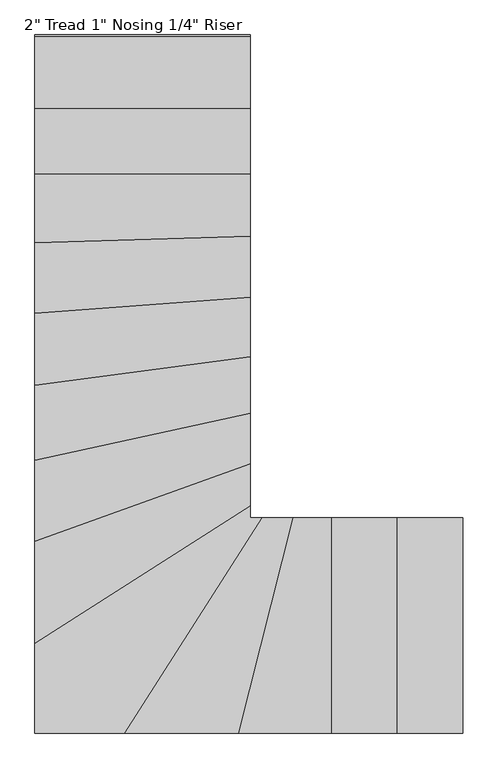
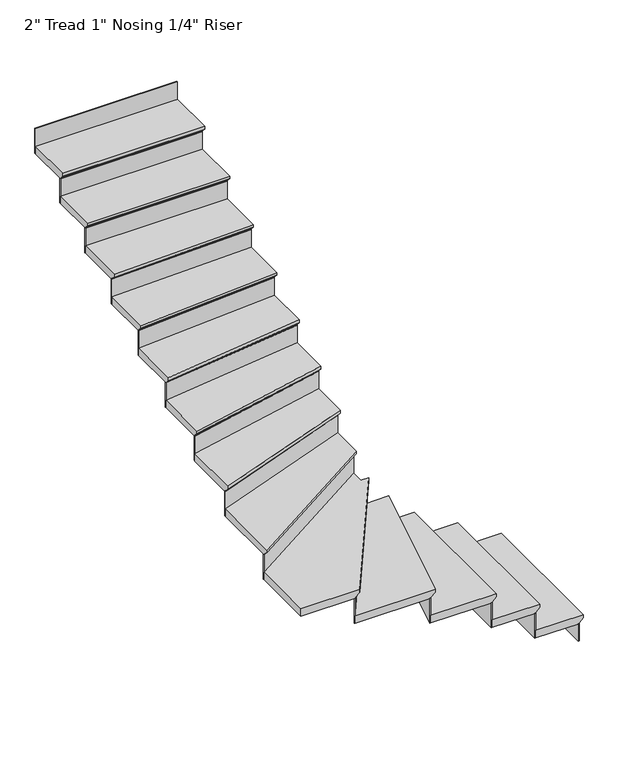
"""IFC4 building model written with IfcOpenShell, lengths in millimetres: stair flight geometry."""

from ifc_helpers import new_model, si_unit, origin, place, context, project, spatial, faceted_brep, source, transform, mapped, element, save


def stair_flight_28aaa101(model_context):
    return source(origin(), model_context, "Body", "Brep", [
        faceted_brep([(-12359.4290643, 4794.153629, 827.6166667), (-12359.4290643, 4794.153629, 846.6666667), (-12359.4290643, 3879.753629, 846.6666667), (-12359.4290643, 3879.753629, 827.6166667), (-12384.8290643, 4794.153629, 802.2166667), (-12384.8290643, 3879.753629, 802.2166667), (-12664.2290643, 4794.153629, 846.6666667), (-12664.2290643, 3879.753629, 846.6666667), (-12384.8290643, 3879.753629, 795.8666667), (-12664.2290643, 3879.753629, 795.8666667), (-12664.2290643, 4794.153629, 795.8666667), (-12384.8290643, 4794.153629, 795.8666667)], [[[0, 1, 2, 3]], [[4, 0, 3, 5]], [[2, 1, 6, 7]], [[8, 9, 10, 11]], [[2, 7, 9, 8, 5, 3]], [[8, 11, 4, 5]], [[6, 1, 0, 4, 11, 10]], [[7, 6, 10, 9]]]),
        faceted_brep([(-12384.8290643, 4794.153629, 795.8666667), (-12384.8290643, 4794.153629, 677.3333333), (-12391.1790643, 4794.153629, 677.3333333), (-12391.1790643, 4794.153629, 795.8666667), (-12384.8290643, 3879.753629, 795.8666667), (-12391.1790643, 3879.753629, 795.8666667), (-12391.1790643, 3879.753629, 677.3333333), (-12384.8290643, 3879.753629, 677.3333333)], [[[0, 1, 2, 3]], [[4, 5, 6, 7]], [[1, 0, 4, 7]], [[2, 1, 7, 6]], [[3, 2, 6, 5]], [[0, 3, 5, 4]]]),
        faceted_brep([(-12664.2290643, 4794.153629, 965.2), (-12664.2290643, 4794.153629, 795.8666667), (-12670.5790643, 4794.153629, 795.8666667), (-12670.5790643, 4794.153629, 965.2), (-12664.2290643, 3879.753629, 965.2), (-12670.5790643, 3879.753629, 965.2), (-12670.5790643, 3879.753629, 795.8666667), (-12664.2290643, 3879.753629, 795.8666667)], [[[0, 1, 2, 3]], [[4, 5, 6, 7]], [[1, 0, 4, 7]], [[2, 1, 7, 6]], [[3, 2, 6, 5]], [[0, 3, 5, 4]]]),
        faceted_brep([(-12638.8290643, 3879.753629, 1016.0), (-12638.8290643, 4794.153629, 1016.0), (-12943.6290643, 4794.153629, 1016.0), (-12943.6290643, 3879.753629, 1016.0), (-12664.2290643, 3879.753629, 965.2), (-12943.6290643, 3879.753629, 965.2), (-12943.6290643, 4794.153629, 965.2), (-12664.2290643, 4794.153629, 965.2), (-12664.2290643, 3879.753629, 971.55), (-12638.8290643, 3879.753629, 996.95), (-12664.2290643, 4794.153629, 971.55), (-12638.8290643, 4794.153629, 996.95)], [[[0, 1, 2, 3]], [[4, 5, 6, 7]], [[0, 3, 5, 4, 8, 9]], [[4, 7, 10, 8]], [[2, 1, 11, 10, 7, 6]], [[3, 2, 6, 5]], [[11, 1, 0, 9]], [[10, 11, 9, 8]]]),
        faceted_brep([(-12943.6290643, 4794.153629, 1134.5333333), (-12943.6290643, 4794.153629, 965.2), (-12949.9790643, 4794.153629, 965.2), (-12949.9790643, 4794.153629, 1134.5333333), (-12943.6290643, 3879.753629, 1134.5333333), (-12949.9790643, 3879.753629, 1134.5333333), (-12949.9790643, 3879.753629, 965.2), (-12943.6290643, 3879.753629, 965.2)], [[[0, 1, 2, 3]], [[4, 5, 6, 7]], [[1, 0, 4, 7]], [[2, 1, 7, 6]], [[3, 2, 6, 5]], [[0, 3, 5, 4]]]),
        faceted_brep([(-12918.2290643, 3879.753629, 1185.3333333), (-12918.2290643, 4794.153629, 1185.3333333), (-13108.3340982, 4794.153629, 1185.3333333), (-13339.3197748, 3879.753629, 1185.3333333), (-12943.6290643, 3879.753629, 1134.5333333), (-13339.3197748, 3879.753629, 1134.5333333), (-13108.3340982, 4794.153629, 1134.5333333), (-12943.6290643, 4794.153629, 1134.5333333), (-12943.6290643, 3879.753629, 1140.8833333), (-12918.2290643, 3879.753629, 1166.2833333), (-12943.6290643, 4794.153629, 1140.8833333), (-12918.2290643, 4794.153629, 1166.2833333)], [[[0, 1, 2, 3]], [[4, 5, 6, 7]], [[0, 3, 5, 4, 8, 9]], [[4, 7, 10, 8]], [[2, 1, 11, 10, 7, 6]], [[3, 2, 6, 5]], [[11, 1, 0, 9]], [[10, 11, 9, 8]]]),
        faceted_brep([(-13108.3340982, 4794.153629, 1303.8666667), (-13108.3340982, 4794.153629, 1134.5333333), (-13114.8835662, 4794.153629, 1134.5333333), (-13114.8835662, 4794.153629, 1303.8666667), (-13339.3197748, 3879.753629, 1303.8666667), (-13345.8692428, 3879.753629, 1303.8666667), (-13345.8692428, 3879.753629, 1134.5333333), (-13339.3197748, 3879.753629, 1134.5333333)], [[[0, 1, 2, 3]], [[4, 5, 6, 7]], [[1, 0, 4, 7]], [[2, 1, 7, 6]], [[3, 2, 6, 5]], [[0, 3, 5, 4]]]),
        faceted_brep([(-13313.1219026, 3879.753629, 1354.6666667), (-13082.136226, 4794.153629, 1354.6666667), (-13242.6016872, 4794.153629, 1354.6666667), (-13827.2011226, 3879.753629, 1354.6666667), (-13339.3197748, 3879.753629, 1303.8666667), (-13827.2011226, 3879.753629, 1303.8666667), (-13242.6016872, 4794.153629, 1303.8666667), (-13108.3340982, 4794.153629, 1303.8666667), (-13339.3197748, 3879.753629, 1310.2166667), (-13313.1219026, 3879.753629, 1335.6166667), (-13108.3340982, 4794.153629, 1310.2166667), (-13082.136226, 4794.153629, 1335.6166667)], [[[0, 1, 2, 3]], [[4, 5, 6, 7]], [[0, 3, 5, 4, 8, 9]], [[4, 7, 10, 8]], [[2, 1, 11, 10, 7, 6]], [[3, 2, 6, 5]], [[11, 1, 0, 9]], [[10, 11, 9, 8]]]),
        faceted_brep([(-13242.6016872, 4794.153629, 1473.2), (-13242.6016872, 4794.153629, 1303.8666667), (-13250.1385176, 4794.153629, 1303.8666667), (-13250.1385176, 4794.153629, 1473.2), (-13827.2011226, 3879.753629, 1473.2), (-13834.737953, 3879.753629, 1473.2), (-13834.737953, 3879.753629, 1303.8666667), (-13827.2011226, 3879.753629, 1303.8666667)], [[[0, 1, 2, 3]], [[4, 5, 6, 7]], [[1, 0, 4, 7]], [[2, 1, 7, 6]], [[3, 2, 6, 5]], [[0, 3, 5, 4]]]),
        faceted_brep([(-14177.7660538, 4290.6132035, 1524.0), (-14177.7660538, 3879.753629, 1524.0), (-13797.053801, 3879.753629, 1524.0), (-13212.4543656, 4794.153629, 1524.0), (-13263.3660538, 4794.153629, 1524.0), (-13263.3660538, 4875.2126389, 1524.0), (-14177.7660538, 3879.753629, 1473.2), (-14177.7660538, 4290.6132035, 1473.2), (-13263.3660538, 4875.2126389, 1473.2), (-13263.3660538, 4794.153629, 1473.2), (-13242.6016872, 4794.153629, 1473.2), (-13827.2011226, 3879.753629, 1473.2), (-13242.6016872, 4794.153629, 1479.55), (-13827.2011226, 3879.753629, 1479.55), (-13212.4543656, 4794.153629, 1504.95), (-13797.053801, 3879.753629, 1504.95)], [[[0, 1, 2, 3, 4, 5]], [[6, 7, 8, 9, 10, 11]], [[1, 0, 7, 6]], [[11, 10, 12, 13]], [[4, 3, 14, 12, 10, 9]], [[0, 5, 8, 7]], [[14, 3, 2, 15]], [[12, 14, 15, 13]], [[2, 1, 6, 11, 13, 15]], [[5, 4, 9, 8]]]),
        faceted_brep([(-13263.3660538, 4875.2126389, 1642.5333333), (-13263.3660538, 4875.2126389, 1473.2), (-13263.3660538, 4882.7494693, 1473.2), (-13263.3660538, 4882.7494693, 1642.5333333), (-14177.7660538, 4290.6132035, 1642.5333333), (-14177.7660538, 4298.1500339, 1642.5333333), (-14177.7660538, 4298.1500339, 1473.2), (-14177.7660538, 4290.6132035, 1473.2)], [[[0, 1, 2, 3]], [[4, 5, 6, 7]], [[1, 0, 4, 7]], [[2, 1, 7, 6]], [[3, 2, 6, 5]], [[0, 3, 5, 4]]]),
        faceted_brep([(-14177.7660538, 4260.4658819, 1693.3333333), (-13263.3660538, 4845.0653173, 1693.3333333), (-13263.3660538, 5051.1689508, 1693.3333333), (-14177.7660538, 4722.592446, 1693.3333333), (-14177.7660538, 4290.6132035, 1642.5333333), (-14177.7660538, 4722.592446, 1642.5333333), (-13263.3660538, 5051.1689508, 1642.5333333), (-13263.3660538, 4875.2126389, 1642.5333333), (-14177.7660538, 4290.6132035, 1648.8833333), (-14177.7660538, 4260.4658819, 1674.2833333), (-13263.3660538, 4875.2126389, 1648.8833333), (-13263.3660538, 4845.0653173, 1674.2833333)], [[[0, 1, 2, 3]], [[4, 5, 6, 7]], [[0, 3, 5, 4, 8, 9]], [[4, 7, 10, 8]], [[2, 1, 11, 10, 7, 6]], [[3, 2, 6, 5]], [[11, 1, 0, 9]], [[10, 11, 9, 8]]]),
        faceted_brep([(-13263.3660538, 5051.1689508, 1811.8666667), (-13263.3660538, 5051.1689508, 1642.5333333), (-13263.3660538, 5057.9164708, 1642.5333333), (-13263.3660538, 5057.9164708, 1811.8666667), (-14177.7660538, 4722.592446, 1811.8666667), (-14177.7660538, 4729.339966, 1811.8666667), (-14177.7660538, 4729.339966, 1642.5333333), (-14177.7660538, 4722.592446, 1642.5333333)], [[[0, 1, 2, 3]], [[4, 5, 6, 7]], [[1, 0, 4, 7]], [[2, 1, 7, 6]], [[3, 2, 6, 5]], [[0, 3, 5, 4]]]),
        faceted_brep([(-14177.7660538, 4695.6023661, 1862.6666667), (-13263.3660538, 5024.1788709, 1862.6666667), (-13263.3660538, 5265.2853499, 1862.6666667), (-14177.7660538, 5065.2966833, 1862.6666667), (-14177.7660538, 4722.592446, 1811.8666667), (-14177.7660538, 5065.2966833, 1811.8666667), (-13263.3660538, 5265.2853499, 1811.8666667), (-13263.3660538, 5051.1689508, 1811.8666667), (-14177.7660538, 4722.592446, 1818.2166667), (-14177.7660538, 4695.6023661, 1843.6166667), (-13263.3660538, 5051.1689508, 1818.2166667), (-13263.3660538, 5024.1788709, 1843.6166667)], [[[0, 1, 2, 3]], [[4, 5, 6, 7]], [[0, 3, 5, 4, 8, 9]], [[4, 7, 10, 8]], [[2, 1, 11, 10, 7, 6]], [[3, 2, 6, 5]], [[11, 1, 0, 9]], [[10, 11, 9, 8]]]),
        faceted_brep([(-13263.3660538, 5265.2853499, 1981.2), (-13263.3660538, 5265.2853499, 1811.8666667), (-13263.3660538, 5271.7854494, 1811.8666667), (-13263.3660538, 5271.7854494, 1981.2), (-14177.7660538, 5065.2966833, 1981.2), (-14177.7660538, 5071.7967828, 1981.2), (-14177.7660538, 5071.7967828, 1811.8666667), (-14177.7660538, 5065.2966833, 1811.8666667)], [[[0, 1, 2, 3]], [[4, 5, 6, 7]], [[1, 0, 4, 7]], [[2, 1, 7, 6]], [[3, 2, 6, 5]], [[0, 3, 5, 4]]]),
        faceted_brep([(-14177.7660538, 5039.2962852, 2032.0), (-13263.3660538, 5239.2849518, 2032.0), (-13263.3660538, 5504.83239, 2032.0), (-14177.7660538, 5383.7919779, 2032.0), (-14177.7660538, 5065.2966833, 1981.2), (-14177.7660538, 5383.7919779, 1981.2), (-13263.3660538, 5504.83239, 1981.2), (-13263.3660538, 5265.2853499, 1981.2), (-14177.7660538, 5065.2966833, 1987.55), (-14177.7660538, 5039.2962852, 2012.95), (-13263.3660538, 5265.2853499, 1987.55), (-13263.3660538, 5239.2849518, 2012.95)], [[[0, 1, 2, 3]], [[4, 5, 6, 7]], [[0, 3, 5, 4, 8, 9]], [[4, 7, 10, 8]], [[2, 1, 11, 10, 7, 6]], [[3, 2, 6, 5]], [[11, 1, 0, 9]], [[10, 11, 9, 8]]]),
        faceted_brep([(-13263.3660538, 5504.83239, 2150.5333333), (-13263.3660538, 5504.83239, 1981.2), (-13263.3660538, 5511.2377813, 1981.2), (-13263.3660538, 5511.2377813, 2150.5333333), (-14177.7660538, 5383.7919779, 2150.5333333), (-14177.7660538, 5390.1973693, 2150.5333333), (-14177.7660538, 5390.1973693, 1981.2), (-14177.7660538, 5383.7919779, 1981.2)], [[[0, 1, 2, 3]], [[4, 5, 6, 7]], [[1, 0, 4, 7]], [[2, 1, 7, 6]], [[3, 2, 6, 5]], [[0, 3, 5, 4]]]),
        faceted_brep([(-14177.7660538, 5358.1704125, 2201.3333333), (-13263.3660538, 5479.2108246, 2201.3333333), (-13263.3660538, 5757.3791148, 2201.3333333), (-14177.7660538, 5689.7409105, 2201.3333333), (-14177.7660538, 5383.7919779, 2150.5333333), (-14177.7660538, 5689.7409105, 2150.5333333), (-13263.3660538, 5757.3791148, 2150.5333333), (-13263.3660538, 5504.83239, 2150.5333333), (-14177.7660538, 5383.7919779, 2156.8833333), (-14177.7660538, 5358.1704125, 2182.2833333), (-13263.3660538, 5504.83239, 2156.8833333), (-13263.3660538, 5479.2108246, 2182.2833333)], [[[0, 1, 2, 3]], [[4, 5, 6, 7]], [[0, 3, 5, 4, 8, 9]], [[4, 7, 10, 8]], [[2, 1, 11, 10, 7, 6]], [[3, 2, 6, 5]], [[11, 1, 0, 9]], [[10, 11, 9, 8]]]),
        faceted_brep([(-13263.3660538, 5757.3791148, 2319.8666667), (-13263.3660538, 5757.3791148, 2150.5333333), (-13263.3660538, 5763.7464633, 2150.5333333), (-13263.3660538, 5763.7464633, 2319.8666667), (-14177.7660538, 5689.7409105, 2319.8666667), (-14177.7660538, 5696.108259, 2319.8666667), (-14177.7660538, 5696.108259, 2150.5333333), (-14177.7660538, 5689.7409105, 2150.5333333)], [[[0, 1, 2, 3]], [[4, 5, 6, 7]], [[1, 0, 4, 7]], [[2, 1, 7, 6]], [[3, 2, 6, 5]], [[0, 3, 5, 4]]]),
        faceted_brep([(-14177.7660538, 5664.2715164, 2370.6666667), (-13263.3660538, 5731.9097207, 2370.6666667), (-13263.3660538, 6017.458228, 2370.6666667), (-14177.7660538, 5988.3487438, 2370.6666667), (-14177.7660538, 5689.7409105, 2319.8666667), (-14177.7660538, 5988.3487438, 2319.8666667), (-13263.3660538, 6017.458228, 2319.8666667), (-13263.3660538, 5757.3791148, 2319.8666667), (-14177.7660538, 5689.7409105, 2326.2166667), (-14177.7660538, 5664.2715164, 2351.6166667), (-13263.3660538, 5757.3791148, 2326.2166667), (-13263.3660538, 5731.9097207, 2351.6166667)], [[[0, 1, 2, 3]], [[4, 5, 6, 7]], [[0, 3, 5, 4, 8, 9]], [[4, 7, 10, 8]], [[2, 1, 11, 10, 7, 6]], [[3, 2, 6, 5]], [[11, 1, 0, 9]], [[10, 11, 9, 8]]]),
        faceted_brep([(-13263.3660538, 6017.458228, 2489.2), (-13263.3660538, 6017.458228, 2319.8666667), (-13263.3660538, 6023.8114448, 2319.8666667), (-13263.3660538, 6023.8114448, 2489.2), (-14177.7660538, 5988.3487438, 2489.2), (-14177.7660538, 5994.7019607, 2489.2), (-14177.7660538, 5994.7019607, 2319.8666667), (-14177.7660538, 5988.3487438, 2319.8666667)], [[[0, 1, 2, 3]], [[4, 5, 6, 7]], [[1, 0, 4, 7]], [[2, 1, 7, 6]], [[3, 2, 6, 5]], [[0, 3, 5, 4]]]),
        faceted_brep([(-14177.7660538, 5962.9358765, 2540.0), (-13263.3660538, 5992.0453606, 2540.0), (-13263.3660538, 6282.2906185, 2540.0), (-14177.7660538, 6282.2906185, 2540.0), (-14177.7660538, 5988.3487438, 2489.2), (-14177.7660538, 6282.2906185, 2489.2), (-13263.3660538, 6282.2906185, 2489.2), (-13263.3660538, 6017.458228, 2489.2), (-14177.7660538, 5988.3487438, 2495.55), (-14177.7660538, 5962.9358765, 2520.95), (-13263.3660538, 6017.458228, 2495.55), (-13263.3660538, 5992.0453606, 2520.95)], [[[0, 1, 2, 3]], [[4, 5, 6, 7]], [[0, 3, 5, 4, 8, 9]], [[4, 7, 10, 8]], [[2, 1, 11, 10, 7, 6]], [[3, 2, 6, 5]], [[11, 1, 0, 9]], [[10, 11, 9, 8]]]),
        faceted_brep([(-13263.3660538, 6282.2906185, 2658.5333333), (-13263.3660538, 6282.2906185, 2489.2), (-13263.3660538, 6288.6406185, 2489.2), (-13263.3660538, 6288.6406185, 2658.5333333), (-14177.7660538, 6282.2906185, 2658.5333333), (-14177.7660538, 6288.6406185, 2658.5333333), (-14177.7660538, 6288.6406185, 2489.2), (-14177.7660538, 6282.2906185, 2489.2)], [[[0, 1, 2, 3]], [[4, 5, 6, 7]], [[1, 0, 4, 7]], [[2, 1, 7, 6]], [[3, 2, 6, 5]], [[0, 3, 5, 4]]]),
        faceted_brep([(-14177.7660538, 6256.8906185, 2709.3333333), (-13263.3660538, 6256.8906185, 2709.3333333), (-13263.3660538, 6561.6906185, 2709.3333333), (-14177.7660538, 6561.6906185, 2709.3333333), (-14177.7660538, 6282.2906185, 2658.5333333), (-14177.7660538, 6561.6906185, 2658.5333333), (-13263.3660538, 6561.6906185, 2658.5333333), (-13263.3660538, 6282.2906185, 2658.5333333), (-14177.7660538, 6282.2906185, 2664.8833333), (-14177.7660538, 6256.8906185, 2690.2833333), (-13263.3660538, 6282.2906185, 2664.8833333), (-13263.3660538, 6256.8906185, 2690.2833333)], [[[0, 1, 2, 3]], [[4, 5, 6, 7]], [[0, 3, 5, 4, 8, 9]], [[4, 7, 10, 8]], [[2, 1, 11, 10, 7, 6]], [[3, 2, 6, 5]], [[11, 1, 0, 9]], [[10, 11, 9, 8]]]),
        faceted_brep([(-13263.3660538, 6561.6906185, 2827.8666667), (-13263.3660538, 6561.6906185, 2658.5333333), (-13263.3660538, 6568.0406185, 2658.5333333), (-13263.3660538, 6568.0406185, 2827.8666667), (-14177.7660538, 6561.6906185, 2827.8666667), (-14177.7660538, 6568.0406185, 2827.8666667), (-14177.7660538, 6568.0406185, 2658.5333333), (-14177.7660538, 6561.6906185, 2658.5333333)], [[[0, 1, 2, 3]], [[4, 5, 6, 7]], [[1, 0, 4, 7]], [[2, 1, 7, 6]], [[3, 2, 6, 5]], [[0, 3, 5, 4]]]),
        faceted_brep([(-13263.3660538, 6841.0906185, 2997.2), (-13263.3660538, 6841.0906185, 2827.8666667), (-13263.3660538, 6847.4406185, 2827.8666667), (-13263.3660538, 6847.4406185, 2997.2), (-14177.7660538, 6841.0906185, 2997.2), (-14177.7660538, 6847.4406185, 2997.2), (-14177.7660538, 6847.4406185, 2827.8666667), (-14177.7660538, 6841.0906185, 2827.8666667)], [[[0, 1, 2, 3]], [[4, 5, 6, 7]], [[1, 0, 4, 7]], [[2, 1, 7, 6]], [[3, 2, 6, 5]], [[0, 3, 5, 4]]]),
        faceted_brep([(-14177.7660538, 6536.2906185, 2878.6666667), (-13263.3660538, 6536.2906185, 2878.6666667), (-13263.3660538, 6841.0906185, 2878.6666667), (-14177.7660538, 6841.0906185, 2878.6666667), (-14177.7660538, 6561.6906185, 2827.8666667), (-14177.7660538, 6841.0906185, 2827.8666667), (-13263.3660538, 6841.0906185, 2827.8666667), (-13263.3660538, 6561.6906185, 2827.8666667), (-14177.7660538, 6561.6906185, 2834.2166667), (-14177.7660538, 6536.2906185, 2859.6166667), (-13263.3660538, 6561.6906185, 2834.2166667), (-13263.3660538, 6536.2906185, 2859.6166667)], [[[0, 1, 2, 3]], [[4, 5, 6, 7]], [[0, 3, 5, 4, 8, 9]], [[4, 7, 10, 8]], [[2, 1, 11, 10, 7, 6]], [[3, 2, 6, 5]], [[11, 1, 0, 9]], [[10, 11, 9, 8]]]),
    ])


if __name__ == "__main__":
    model = new_model("IFC4")
    model_context = context("Model", 3, world=origin())
    ifc_project = project(units=[si_unit("LENGTHUNIT", "METRE", prefix="MILLI")], contexts=[model_context])
    site = spatial("IfcSite", under=ifc_project)
    building = spatial("IfcBuilding", under=site)
    placement = place(None, origin())
    stair_flight_shape = stair_flight_28aaa101(model_context)
    element("IfcStairFlight", 1, ObjectType="2\" Tread 1\" Nosing 1/4\" Riser", at=placement, inside=building, context=model_context, shape_type="MappedRepresentation", body=[
        mapped(stair_flight_shape, transform((0.0, 0.0, 0.0), x_axis=(1.0, 0.0, 0.0), y_axis=(0.0, 1.0, 0.0), z_axis=(0.0, 0.0, 1.0))),
    ])
    save(model, "model.ifc")
